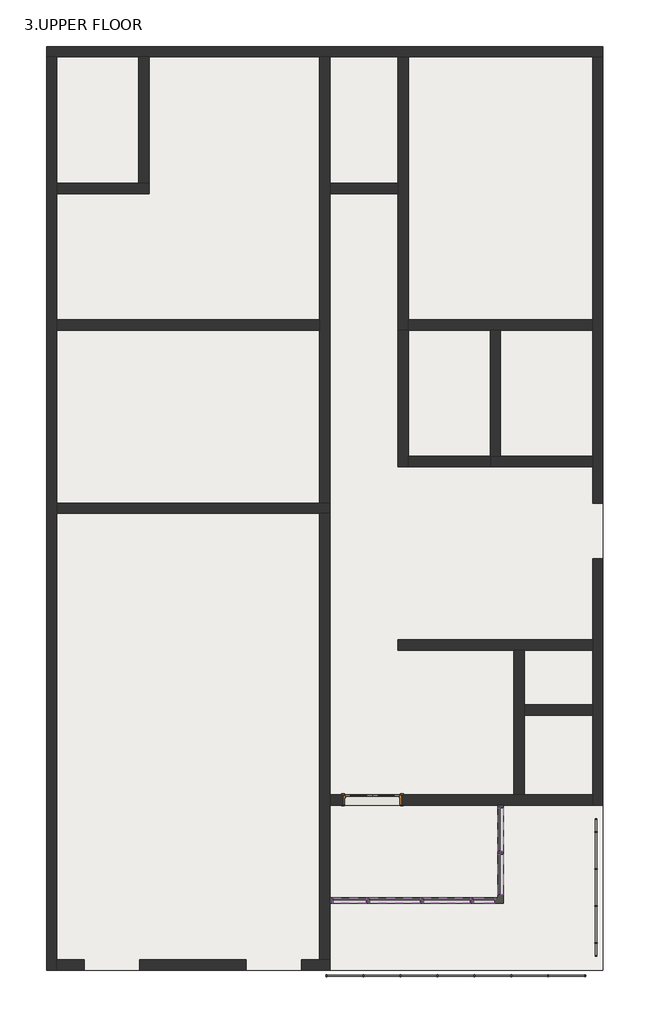
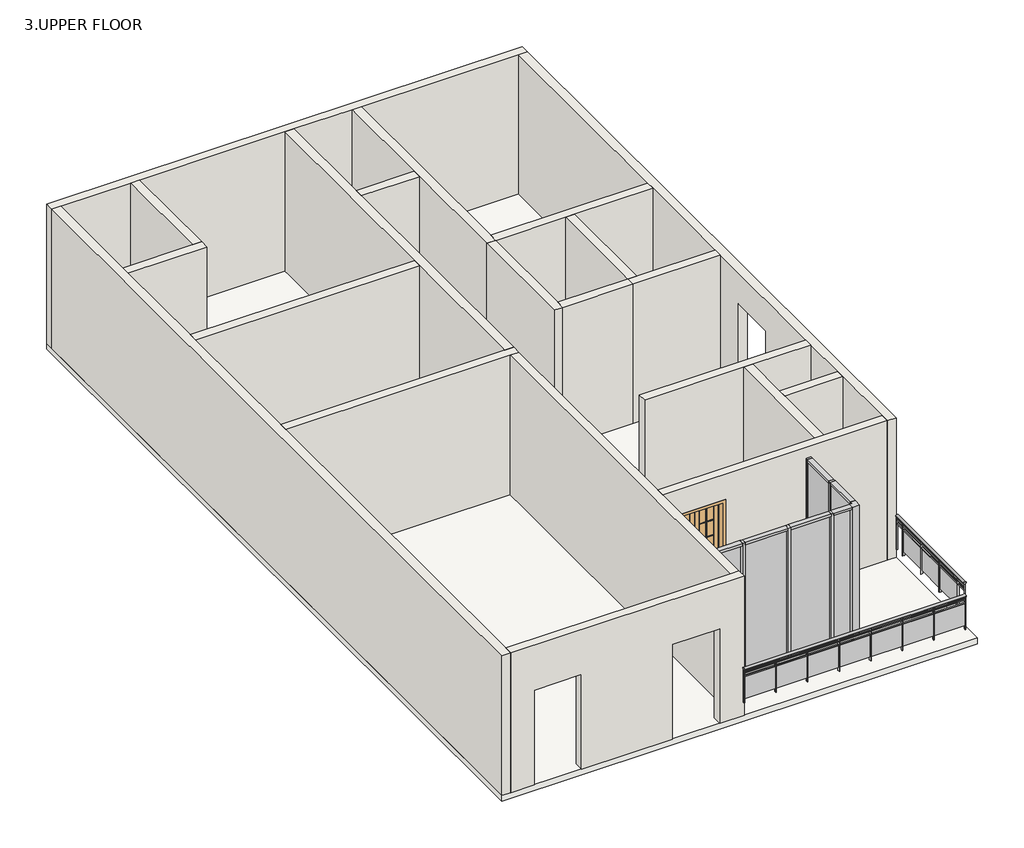
# One storey: 21 walls, 19 members, 6 plates, 2 railings, 1 door, 1 slab.
"""IFC4 building model written with IfcOpenShell, lengths in millimetres."""

from ifc_helpers import new_model, si_unit, point, frame, origin, place, context, project, spatial, polyline, ellipse_curve, trimmed, outline, extrude, faceted_brep, transform, mapped, element, save
from ifc_brep_helpers import plane_surface, extruded_surface, advanced_brep
from components import door_interior_double_full_glass_wood_4_x_8_0c92ad92, member_693e8272, member_0ce7375f, member_58dfa4c6, member_05798353, member_3e299884, member_a8ebf488, member_6e66df9c, member_e4ba5a11, member_9cf8e2d9, system_panel_glazed_02167798, system_panel_glazed_3d2c66d7, system_panel_glazed_0d5058d0, system_panel_glazed_5332cc33, system_panel_glazed_aeaff5c2, system_panel_glazed_b03b416e

model = new_model("IFC4")

# Units and contexts
model_context = context("Model", 3, world=origin())
ifc_project = project(units=[si_unit("LENGTHUNIT", "METRE", prefix="MILLI")], contexts=[model_context])

# Site, building, storey
site = spatial("IfcSite", under=ifc_project)
building = spatial("IfcBuilding", under=site)
storey = spatial("IfcBuildingStorey", under=building, Name="3.UPPER FLOOR", Elevation=3750.0)

# Door
placement = place(None, origin())
door_interior_double_full_glass_wood_4_x_8_shape = door_interior_double_full_glass_wood_4_x_8_0c92ad92(model_context)
element("IfcDoor", 1, ObjectType="Door-Interior-Double-Full Glass-Wood : 4' x 8'", at=placement, inside=storey, context=model_context, shape_type="MappedRepresentation", body=[
    mapped(door_interior_double_full_glass_wood_4_x_8_shape, transform((825.5463749, -5959.698087, 4359.6), x_axis=(1.0, 0.0, 0.0), y_axis=(0.0, 1.0, 0.0), z_axis=(0.0, 0.0, 1.0))),
])

# Members
member_shape = member_693e8272(model_context)
element("IfcMember", 2, ObjectType="L Corner Mullion : 5\" x 5\" Corner", at=placement, inside=storey, context=model_context, shape_type="MappedRepresentation", body=[
    mapped(member_shape, transform((3644.1463749, -8174.973087, 3750.0), x_axis=(1.0, 0.0, 0.0), y_axis=(0.0, -1.0, 0.0), z_axis=(0.0, 0.0, -1.0))),
])
member_2_shape = member_0ce7375f(model_context)
element("IfcMember", 3, ObjectType="Rectangular Mullion : 2.5\" x 5\" rectangular", at=placement, inside=storey, context=model_context, shape_type="MappedRepresentation", body=[
    mapped(member_2_shape, transform((-45.9536251, -8174.973087, 3750.0), x_axis=(0.0, 0.0, -1.0), y_axis=(0.0, -1.0, 0.0), z_axis=(-1.0, 0.0, 0.0))),
])
member_3_shape = member_58dfa4c6(model_context)
element("IfcMember", 4, ObjectType="Rectangular Mullion : 2.5\" x 5\" rectangular", at=placement, inside=storey, context=model_context, shape_type="MappedRepresentation", body=[
    mapped(member_3_shape, transform((730.5463749, -8174.973087, 3750.0), x_axis=(1.0, 0.0, 0.0), y_axis=(0.0, -1.0, 0.0), z_axis=(0.0, 0.0, -1.0))),
])
element("IfcMember", 5, ObjectType="Rectangular Mullion : 2.5\" x 5\" rectangular", at=placement, inside=storey, context=model_context, shape_type="MappedRepresentation", body=[
    mapped(member_3_shape, transform((1910.5463749, -8174.973087, 3750.0), x_axis=(1.0, 0.0, 0.0), y_axis=(0.0, -1.0, 0.0), z_axis=(0.0, 0.0, -1.0))),
])
element("IfcMember", 6, ObjectType="Rectangular Mullion : 2.5\" x 5\" rectangular", at=placement, inside=storey, context=model_context, shape_type="MappedRepresentation", body=[
    mapped(member_3_shape, transform((3012.9463749, -8174.973087, 3750.0), x_axis=(1.0, 0.0, 0.0), y_axis=(0.0, -1.0, 0.0), z_axis=(0.0, 0.0, -1.0))),
])
element("IfcMember", 7, ObjectType="Rectangular Mullion : 2.5\" x 5\" rectangular", at=placement, inside=storey, context=model_context, shape_type="MappedRepresentation", body=[
    mapped(member_3_shape, transform((3644.1463749, -7126.073087, 3750.0), x_axis=(0.0, 1.0, 0.0), y_axis=(1.0, 0.0, 0.0), z_axis=(0.0, 0.0, -1.0))),
])
member_4_shape = member_05798353(model_context)
element("IfcMember", 8, ObjectType="Rectangular Mullion : 2.5\" x 5\" rectangular", at=placement, inside=storey, context=model_context, shape_type="MappedRepresentation", body=[
    mapped(member_4_shape, transform((762.2963749, -8174.973087, 3750.0), x_axis=(0.0, 0.0, -1.0), y_axis=(0.0, -1.0, 0.0), z_axis=(-1.0, 0.0, 0.0))),
])
member_5_shape = member_3e299884(model_context)
element("IfcMember", 9, ObjectType="Rectangular Mullion : 2.5\" x 5\" rectangular", at=placement, inside=storey, context=model_context, shape_type="MappedRepresentation", body=[
    mapped(member_5_shape, transform((1942.2963749, -8174.973087, 3750.0), x_axis=(0.0, 0.0, -1.0), y_axis=(0.0, -1.0, 0.0), z_axis=(-1.0, 0.0, 0.0))),
])
element("IfcMember", 10, ObjectType="Rectangular Mullion : 2.5\" x 5\" rectangular", at=placement, inside=storey, context=model_context, shape_type="MappedRepresentation", body=[
    mapped(member_2_shape, transform((698.7963749, -8174.973087, 7256.9820397), x_axis=(0.0, 0.0, 1.0), y_axis=(0.0, -1.0, 0.0), z_axis=(1.0, 0.0, 0.0))),
])
element("IfcMember", 11, ObjectType="Rectangular Mullion : 2.5\" x 5\" rectangular", at=placement, inside=storey, context=model_context, shape_type="MappedRepresentation", body=[
    mapped(member_4_shape, transform((1878.7963749, -8174.973087, 7256.9820397), x_axis=(0.0, 0.0, 1.0), y_axis=(0.0, -1.0, 0.0), z_axis=(1.0, 0.0, 0.0))),
])
element("IfcMember", 12, ObjectType="Rectangular Mullion : 2.5\" x 5\" rectangular", at=placement, inside=storey, context=model_context, shape_type="MappedRepresentation", body=[
    mapped(member_5_shape, transform((2981.1963749, -8174.973087, 7256.9820397), x_axis=(0.0, 0.0, 1.0), y_axis=(0.0, -1.0, 0.0), z_axis=(1.0, 0.0, 0.0))),
])
member_6_shape = member_a8ebf488(model_context)
element("IfcMember", 13, ObjectType="Rectangular Mullion : 2.5\" x 5\" rectangular", at=placement, inside=storey, context=model_context, shape_type="MappedRepresentation", body=[
    mapped(member_6_shape, transform((-109.4536251, -8174.973087, 7256.9820397), x_axis=(-1.0, 0.0, 0.0), y_axis=(0.0, -1.0, 0.0), z_axis=(0.0, 0.0, 1.0))),
])
element("IfcMember", 14, ObjectType="Rectangular Mullion : 2.5\" x 5\" rectangular", at=placement, inside=storey, context=model_context, shape_type="MappedRepresentation", body=[
    mapped(member_6_shape, transform((3644.1463749, -6077.173087, 3750.0), x_axis=(0.0, 1.0, 0.0), y_axis=(1.0, 0.0, 0.0), z_axis=(0.0, 0.0, -1.0))),
])
member_7_shape = member_6e66df9c(model_context)
element("IfcMember", 15, ObjectType="Rectangular Mullion : 2.5\" x 5\" rectangular", at=placement, inside=storey, context=model_context, shape_type="MappedRepresentation", body=[
    mapped(member_7_shape, transform((3644.1463749, -6140.673087, 7256.9820397), x_axis=(0.0, 0.0, 1.0), y_axis=(1.0, 0.0, 0.0), z_axis=(0.0, 1.0, 0.0))),
])
element("IfcMember", 16, ObjectType="Rectangular Mullion : 2.5\" x 5\" rectangular", at=placement, inside=storey, context=model_context, shape_type="MappedRepresentation", body=[
    mapped(member_7_shape, transform((3644.1463749, -7094.323087, 3750.0), x_axis=(0.0, 0.0, -1.0), y_axis=(1.0, 0.0, 0.0), z_axis=(0.0, -1.0, 0.0))),
])
member_8_shape = member_e4ba5a11(model_context)
element("IfcMember", 17, ObjectType="Rectangular Mullion : 2.5\" x 5\" rectangular", at=placement, inside=storey, context=model_context, shape_type="MappedRepresentation", body=[
    mapped(member_8_shape, transform((3517.1463749, -8174.973087, 7256.9820397), x_axis=(0.0, 0.0, 1.0), y_axis=(0.0, -1.0, 0.0), z_axis=(1.0, 0.0, 0.0))),
])
element("IfcMember", 18, ObjectType="Rectangular Mullion : 2.5\" x 5\" rectangular", at=placement, inside=storey, context=model_context, shape_type="MappedRepresentation", body=[
    mapped(member_8_shape, transform((3044.6963749, -8174.973087, 3750.0), x_axis=(0.0, 0.0, -1.0), y_axis=(0.0, -1.0, 0.0), z_axis=(-1.0, 0.0, 0.0))),
])
member_9_shape = member_9cf8e2d9(model_context)
element("IfcMember", 19, ObjectType="Rectangular Mullion : 2.5\" x 5\" rectangular", at=placement, inside=storey, context=model_context, shape_type="MappedRepresentation", body=[
    mapped(member_9_shape, transform((3644.1463749, -8047.973087, 3750.0), x_axis=(0.0, 0.0, -1.0), y_axis=(1.0, 0.0, 0.0), z_axis=(0.0, -1.0, 0.0))),
])
element("IfcMember", 20, ObjectType="Rectangular Mullion : 2.5\" x 5\" rectangular", at=placement, inside=storey, context=model_context, shape_type="MappedRepresentation", body=[
    mapped(member_9_shape, transform((3644.1463749, -7157.823087, 7256.9820397), x_axis=(0.0, 0.0, 1.0), y_axis=(1.0, 0.0, 0.0), z_axis=(0.0, 1.0, 0.0))),
])

# Plates
system_panel_glazed_shape = system_panel_glazed_02167798(model_context)
element("IfcPlate", 21, ObjectType="System Panel : Glazed", at=placement, inside=storey, context=model_context, shape_type="MappedRepresentation", body=[
    mapped(system_panel_glazed_shape, transform((326.4213749, -8174.973087, 3813.5), x_axis=(1.0, 0.0, 0.0), y_axis=(0.0, 1.0, 0.0), z_axis=(0.0, 0.0, 1.0))),
])
system_panel_glazed_2_shape = system_panel_glazed_3d2c66d7(model_context)
element("IfcPlate", 22, ObjectType="System Panel : Glazed", at=placement, inside=storey, context=model_context, shape_type="MappedRepresentation", body=[
    mapped(system_panel_glazed_2_shape, transform((1320.5463749, -8174.973087, 3813.5), x_axis=(1.0, 0.0, 0.0), y_axis=(0.0, 1.0, 0.0), z_axis=(0.0, 0.0, 1.0))),
])
system_panel_glazed_3_shape = system_panel_glazed_0d5058d0(model_context)
element("IfcPlate", 23, ObjectType="System Panel : Glazed", at=placement, inside=storey, context=model_context, shape_type="MappedRepresentation", body=[
    mapped(system_panel_glazed_3_shape, transform((2461.7463749, -8174.973087, 3813.5), x_axis=(1.0, 0.0, 0.0), y_axis=(0.0, 1.0, 0.0), z_axis=(0.0, 0.0, 1.0))),
])
system_panel_glazed_4_shape = system_panel_glazed_5332cc33(model_context)
element("IfcPlate", 24, ObjectType="System Panel : Glazed", at=placement, inside=storey, context=model_context, shape_type="MappedRepresentation", body=[
    mapped(system_panel_glazed_4_shape, transform((3644.1463749, -6617.498087, 3813.5), x_axis=(0.0, 1.0, 0.0), y_axis=(-1.0, 0.0, 0.0), z_axis=(0.0, 0.0, 1.0))),
])
system_panel_glazed_5_shape = system_panel_glazed_aeaff5c2(model_context)
element("IfcPlate", 25, ObjectType="System Panel : Glazed", at=placement, inside=storey, context=model_context, shape_type="MappedRepresentation", body=[
    mapped(system_panel_glazed_5_shape, transform((3280.9213749, -8174.973087, 3813.5), x_axis=(1.0, 0.0, 0.0), y_axis=(0.0, 1.0, 0.0), z_axis=(0.0, 0.0, 1.0))),
])
system_panel_glazed_6_shape = system_panel_glazed_b03b416e(model_context)
element("IfcPlate", 26, ObjectType="System Panel : Glazed", at=placement, inside=storey, context=model_context, shape_type="MappedRepresentation", body=[
    mapped(system_panel_glazed_6_shape, transform((3644.1463749, -7602.898087, 3813.5), x_axis=(0.0, 1.0, 0.0), y_axis=(-1.0, 0.0, 0.0), z_axis=(0.0, 0.0, 1.0))),
])

# Railings
element("IfcRailing", 27, ObjectType="Glass Panel - Bottom Fill", at=placement, inside=storey, context=model_context, shape_type="SolidModel", body=[
    advanced_brep(
    [(5512.9463749, -9866.673087, 5121.6), (5512.9463749, -9790.473087, 5121.6), (-189.4536251, -9866.673087, 5121.6), (-189.4536251, -9790.473087, 5121.6)],
    [
        (0, 1, ellipse_curve(frame((5512.9463749, -9828.573087, 5121.6), z_axis=(1.0, 0.0, 0.0), x_axis=(0.0, 1.0, 0.0)), 38.1, 28.575)),
        (1, 0, ellipse_curve(frame((5512.9463749, -9828.573087, 5121.6), z_axis=(1.0, 0.0, 0.0), x_axis=(0.0, 1.0, 0.0)), 38.1, 28.575)),
        (2, 3, ellipse_curve(frame((-189.4536251, -9828.573087, 5121.6), z_axis=(-1.0, 0.0, 0.0), x_axis=(0.0, 1.0, 0.0)), 38.1, 28.575)),
        (3, 2, ellipse_curve(frame((-189.4536251, -9828.573087, 5121.6), z_axis=(-1.0, 0.0, 0.0), x_axis=(0.0, 1.0, 0.0)), 38.1, 28.575)),
        (0, 2),
        (3, 1),
    ],
    [
        plane_surface(frame((5512.9463749, -9828.573087, 5121.6), z_axis=(1.0, 0.0, 0.0), x_axis=(0.0, -1.0, 0.0))),
        plane_surface(frame((-189.4536251, -9828.573087, 5121.6), z_axis=(-1.0, 0.0, 0.0), x_axis=(0.0, -1.0, 0.0))),
        extruded_surface(trimmed(ellipse_curve(frame((-189.4536251, -9828.573087, 5121.6), z_axis=(1.0, 0.0, 0.0), x_axis=(0.0, 1.0, 0.0)), 38.1, 28.575), [point((-189.4536251, -9866.673087, 5121.6))], [point((-189.4536251, -9790.473087, 5121.6))], True, "CARTESIAN"), (5702.4, 0.0, 0.0), 5702.4),
        extruded_surface(trimmed(ellipse_curve(frame((-189.4536251, -9828.573087, 5121.6), z_axis=(1.0, 0.0, 0.0), x_axis=(0.0, 1.0, 0.0)), 38.1, 28.575), [point((-189.4536251, -9790.473087, 5121.6))], [point((-189.4536251, -9866.673087, 5121.6))], True, "CARTESIAN"), (5702.4, 0.0, 0.0), 5702.4),
    ],
    [
        (0, [[1, 2]]),
        (1, [[3, 4]]),
        (2, [[-1, 5, -4, 6]]),
        (3, [[-2, -6, -3, -5]]),
    ],
),
    extrude(outline(polyline([(5512.9463749, -9815.873087), (5512.9463749, -9841.273087), (-189.4536251, -9841.273087), (-189.4536251, -9815.873087), (5512.9463749, -9815.873087)])), frame((0.0, 0.0, 5007.3), z_axis=(0.0, 0.0, 1.0), x_axis=(1.0, 0.0, 0.0)), (0.0, 0.0, 1.0), 25.4),
    extrude(outline(polyline([(5512.9463749, -9815.873087), (5512.9463749, -9841.273087), (-189.4536251, -9841.273087), (-189.4536251, -9815.873087), (5512.9463749, -9815.873087)])), frame((0.0, 0.0, 4905.7), z_axis=(0.0, 0.0, 1.0), x_axis=(1.0, 0.0, 0.0)), (0.0, 0.0, 1.0), 25.4),
    extrude(outline(polyline([(-176.7036251, -9803.173087), (-176.7036251, -9853.973087), (-189.4036251, -9853.973087), (-189.4036251, -9803.173087), (-176.7036251, -9803.173087)])), frame((0.0, 0.0, 4207.2), z_axis=(0.0, 0.0, 1.0), x_axis=(1.0, 0.0, 0.0)), (0.0, 0.0, 1.0), 885.825),
    extrude(outline(polyline([(629.7463749, -9835.108244), (-183.0536251, -9835.108244), (-183.0536251, -9828.758244), (629.7463749, -9828.758244), (629.7463749, -9835.108244)])), frame((0.0, 0.0, 4308.8), z_axis=(0.0, 0.0, 1.0), x_axis=(1.0, 0.0, 0.0)), (0.0, 0.0, 1.0), 596.9),
    extrude(outline(polyline([(636.0963749, -9803.173087), (636.0963749, -9853.973087), (623.3963749, -9853.973087), (623.3963749, -9803.173087), (636.0963749, -9803.173087)])), frame((0.0, 0.0, 4207.2), z_axis=(0.0, 0.0, 1.0), x_axis=(1.0, 0.0, 0.0)), (0.0, 0.0, 1.0), 885.825),
    extrude(outline(polyline([(1442.5463749, -9835.108244), (629.7463749, -9835.108244), (629.7463749, -9828.758244), (1442.5463749, -9828.758244), (1442.5463749, -9835.108244)])), frame((0.0, 0.0, 4308.8), z_axis=(0.0, 0.0, 1.0), x_axis=(1.0, 0.0, 0.0)), (0.0, 0.0, 1.0), 596.9),
    extrude(outline(polyline([(1448.8963749, -9803.173087), (1448.8963749, -9853.973087), (1436.1963749, -9853.973087), (1436.1963749, -9803.173087), (1448.8963749, -9803.173087)])), frame((0.0, 0.0, 4207.2), z_axis=(0.0, 0.0, 1.0), x_axis=(1.0, 0.0, 0.0)), (0.0, 0.0, 1.0), 885.825),
    extrude(outline(polyline([(2255.3463749, -9835.108244), (1442.5463749, -9835.108244), (1442.5463749, -9828.758244), (2255.3463749, -9828.758244), (2255.3463749, -9835.108244)])), frame((0.0, 0.0, 4308.8), z_axis=(0.0, 0.0, 1.0), x_axis=(1.0, 0.0, 0.0)), (0.0, 0.0, 1.0), 596.9),
    extrude(outline(polyline([(2261.6963749, -9803.173087), (2261.6963749, -9853.973087), (2248.9963749, -9853.973087), (2248.9963749, -9803.173087), (2261.6963749, -9803.173087)])), frame((0.0, 0.0, 4207.2), z_axis=(0.0, 0.0, 1.0), x_axis=(1.0, 0.0, 0.0)), (0.0, 0.0, 1.0), 885.825),
    extrude(outline(polyline([(3068.1463749, -9835.108244), (2255.3463749, -9835.108244), (2255.3463749, -9828.758244), (3068.1463749, -9828.758244), (3068.1463749, -9835.108244)])), frame((0.0, 0.0, 4308.8), z_axis=(0.0, 0.0, 1.0), x_axis=(1.0, 0.0, 0.0)), (0.0, 0.0, 1.0), 596.9),
    extrude(outline(polyline([(3074.4963749, -9803.173087), (3074.4963749, -9853.973087), (3061.7963749, -9853.973087), (3061.7963749, -9803.173087), (3074.4963749, -9803.173087)])), frame((0.0, 0.0, 4207.2), z_axis=(0.0, 0.0, 1.0), x_axis=(1.0, 0.0, 0.0)), (0.0, 0.0, 1.0), 885.825),
    extrude(outline(polyline([(3880.9463749, -9835.108244), (3068.1463749, -9835.108244), (3068.1463749, -9828.758244), (3880.9463749, -9828.758244), (3880.9463749, -9835.108244)])), frame((0.0, 0.0, 4308.8), z_axis=(0.0, 0.0, 1.0), x_axis=(1.0, 0.0, 0.0)), (0.0, 0.0, 1.0), 596.9),
    extrude(outline(polyline([(3887.2963749, -9803.173087), (3887.2963749, -9853.973087), (3874.5963749, -9853.973087), (3874.5963749, -9803.173087), (3887.2963749, -9803.173087)])), frame((0.0, 0.0, 4207.2), z_axis=(0.0, 0.0, 1.0), x_axis=(1.0, 0.0, 0.0)), (0.0, 0.0, 1.0), 885.825),
    extrude(outline(polyline([(4693.7463749, -9835.108244), (3880.9463749, -9835.108244), (3880.9463749, -9828.758244), (4693.7463749, -9828.758244), (4693.7463749, -9835.108244)])), frame((0.0, 0.0, 4308.8), z_axis=(0.0, 0.0, 1.0), x_axis=(1.0, 0.0, 0.0)), (0.0, 0.0, 1.0), 596.9),
    extrude(outline(polyline([(4700.0963749, -9803.173087), (4700.0963749, -9853.973087), (4687.3963749, -9853.973087), (4687.3963749, -9803.173087), (4700.0963749, -9803.173087)])), frame((0.0, 0.0, 4207.2), z_axis=(0.0, 0.0, 1.0), x_axis=(1.0, 0.0, 0.0)), (0.0, 0.0, 1.0), 885.825),
    extrude(outline(polyline([(5506.5463749, -9835.108244), (4693.7463749, -9835.108244), (4693.7463749, -9828.758244), (5506.5463749, -9828.758244), (5506.5463749, -9835.108244)])), frame((0.0, 0.0, 4308.8), z_axis=(0.0, 0.0, 1.0), x_axis=(1.0, 0.0, 0.0)), (0.0, 0.0, 1.0), 596.9),
    extrude(outline(polyline([(5512.8963749, -9803.173087), (5512.8963749, -9853.973087), (5500.1963749, -9853.973087), (5500.1963749, -9803.173087), (5512.8963749, -9803.173087)])), frame((0.0, 0.0, 4207.2), z_axis=(0.0, 0.0, 1.0), x_axis=(1.0, 0.0, 0.0)), (0.0, 0.0, 1.0), 885.825),
    extrude(outline(polyline([(-176.7536251, -9819.048087), (-176.7536251, -9838.098087), (-195.8036251, -9838.098087), (-195.8036251, -9819.048087), (-176.7536251, -9819.048087)])), frame((0.0, 0.0, 4207.2), z_axis=(0.0, 0.0, 1.0), x_axis=(1.0, 0.0, 0.0)), (0.0, 0.0, 1.0), 885.825),
    extrude(outline(polyline([(5519.2963749, -9819.048087), (5519.2963749, -9838.098087), (5500.2463749, -9838.098087), (5500.2463749, -9819.048087), (5519.2963749, -9819.048087)])), frame((0.0, 0.0, 4207.2), z_axis=(0.0, 0.0, 1.0), x_axis=(1.0, 0.0, 0.0)), (0.0, 0.0, 1.0), 885.825),
])
element("IfcRailing", 28, ObjectType="Glass Panel - Bottom Fill", at=placement, inside=storey, context=model_context, shape_type="SolidModel", body=[
    advanced_brep(
    [(5783.4463749, -6381.973087, 5121.6), (5707.2463749, -6381.973087, 5121.6), (5783.4463749, -9398.773087, 5121.6), (5707.2463749, -9398.773087, 5121.6)],
    [
        (0, 1, ellipse_curve(frame((5745.3463749, -6381.973087, 5121.6), z_axis=(0.0, 1.0, 0.0), x_axis=(-1.0, 0.0, 0.0)), 38.1, 28.575)),
        (1, 0, ellipse_curve(frame((5745.3463749, -6381.973087, 5121.6), z_axis=(0.0, 1.0, 0.0), x_axis=(-1.0, 0.0, 0.0)), 38.1, 28.575)),
        (2, 3, ellipse_curve(frame((5745.3463749, -9398.773087, 5121.6), z_axis=(0.0, -1.0, 0.0), x_axis=(-1.0, 0.0, 0.0)), 38.1, 28.575)),
        (3, 2, ellipse_curve(frame((5745.3463749, -9398.773087, 5121.6), z_axis=(0.0, -1.0, 0.0), x_axis=(-1.0, 0.0, 0.0)), 38.1, 28.575)),
        (0, 2),
        (3, 1),
    ],
    [
        plane_surface(frame((5745.3463749, -6381.973087, 5121.6), z_axis=(0.0, 1.0, 0.0), x_axis=(0.0, 0.0, -1.0))),
        plane_surface(frame((5745.3463749, -9398.773087, 5121.6), z_axis=(0.0, -1.0, 0.0), x_axis=(0.0, 0.0, -1.0))),
        extruded_surface(trimmed(ellipse_curve(frame((5745.3463749, -9398.773087, 5121.6), z_axis=(0.0, 1.0, 0.0), x_axis=(-1.0, 0.0, 0.0)), 38.1, 28.575), [point((5783.4463749, -9398.773087, 5121.6))], [point((5707.2463749, -9398.773087, 5121.6))], True, "CARTESIAN"), (0.0, 3016.7999999999993, 0.0), 3016.7999999999993),
        extruded_surface(trimmed(ellipse_curve(frame((5745.3463749, -9398.773087, 5121.6), z_axis=(0.0, 1.0, 0.0), x_axis=(-1.0, 0.0, 0.0)), 38.1, 28.575), [point((5707.2463749, -9398.773087, 5121.6))], [point((5783.4463749, -9398.773087, 5121.6))], True, "CARTESIAN"), (0.0, 3016.7999999999993, 0.0), 3016.7999999999993),
    ],
    [
        (0, [[1, 2]]),
        (1, [[3, 4]]),
        (2, [[-1, 5, -4, 6]]),
        (3, [[-2, -6, -3, -5]]),
    ],
),
    extrude(outline(polyline([(5732.6463749, -6381.973087), (5758.0463749, -6381.973087), (5758.0463749, -9398.773087), (5732.6463749, -9398.773087), (5732.6463749, -6381.973087)])), frame((0.0, 0.0, 5007.3), z_axis=(0.0, 0.0, 1.0), x_axis=(1.0, 0.0, 0.0)), (0.0, 0.0, 1.0), 25.4),
    extrude(outline(polyline([(5732.6463749, -6381.973087), (5758.0463749, -6381.973087), (5758.0463749, -9398.773087), (5732.6463749, -9398.773087), (5732.6463749, -6381.973087)])), frame((0.0, 0.0, 4905.7), z_axis=(0.0, 0.0, 1.0), x_axis=(1.0, 0.0, 0.0)), (0.0, 0.0, 1.0), 25.4),
    extrude(outline(polyline([(5719.9463749, -9103.223087), (5770.7463749, -9103.223087), (5770.7463749, -9115.923087), (5719.9463749, -9115.923087), (5719.9463749, -9103.223087)])), frame((0.0, 0.0, 4207.2), z_axis=(0.0, 0.0, 1.0), x_axis=(1.0, 0.0, 0.0)), (0.0, 0.0, 1.0), 885.825),
    extrude(outline(polyline([(5751.8815319, -8296.773087), (5751.8815319, -9109.573087), (5745.5315319, -9109.573087), (5745.5315319, -8296.773087), (5751.8815319, -8296.773087)])), frame((0.0, 0.0, 4308.8), z_axis=(0.0, 0.0, 1.0), x_axis=(1.0, 0.0, 0.0)), (0.0, 0.0, 1.0), 596.9),
    extrude(outline(polyline([(5719.9463749, -8290.423087), (5770.7463749, -8290.423087), (5770.7463749, -8303.123087), (5719.9463749, -8303.123087), (5719.9463749, -8290.423087)])), frame((0.0, 0.0, 4207.2), z_axis=(0.0, 0.0, 1.0), x_axis=(1.0, 0.0, 0.0)), (0.0, 0.0, 1.0), 885.825),
    extrude(outline(polyline([(5751.8815319, -7483.973087), (5751.8815319, -8296.773087), (5745.5315319, -8296.773087), (5745.5315319, -7483.973087), (5751.8815319, -7483.973087)])), frame((0.0, 0.0, 4308.8), z_axis=(0.0, 0.0, 1.0), x_axis=(1.0, 0.0, 0.0)), (0.0, 0.0, 1.0), 596.9),
    extrude(outline(polyline([(5719.9463749, -7477.623087), (5770.7463749, -7477.623087), (5770.7463749, -7490.323087), (5719.9463749, -7490.323087), (5719.9463749, -7477.623087)])), frame((0.0, 0.0, 4207.2), z_axis=(0.0, 0.0, 1.0), x_axis=(1.0, 0.0, 0.0)), (0.0, 0.0, 1.0), 885.825),
    extrude(outline(polyline([(5751.8815319, -6671.173087), (5751.8815319, -7483.973087), (5745.5315319, -7483.973087), (5745.5315319, -6671.173087), (5751.8815319, -6671.173087)])), frame((0.0, 0.0, 4308.8), z_axis=(0.0, 0.0, 1.0), x_axis=(1.0, 0.0, 0.0)), (0.0, 0.0, 1.0), 596.9),
    extrude(outline(polyline([(5719.9463749, -6664.823087), (5770.7463749, -6664.823087), (5770.7463749, -6677.523087), (5719.9463749, -6677.523087), (5719.9463749, -6664.823087)])), frame((0.0, 0.0, 4207.2), z_axis=(0.0, 0.0, 1.0), x_axis=(1.0, 0.0, 0.0)), (0.0, 0.0, 1.0), 885.825),
    extrude(outline(polyline([(5735.8213749, -9386.073087), (5754.8713749, -9386.073087), (5754.8713749, -9405.123087), (5735.8213749, -9405.123087), (5735.8213749, -9386.073087)])), frame((0.0, 0.0, 4207.2), z_axis=(0.0, 0.0, 1.0), x_axis=(1.0, 0.0, 0.0)), (0.0, 0.0, 1.0), 885.825),
    extrude(outline(polyline([(5735.8213749, -6375.623087), (5754.8713749, -6375.623087), (5754.8713749, -6394.673087), (5735.8213749, -6394.673087), (5735.8213749, -6375.623087)])), frame((0.0, 0.0, 4207.2), z_axis=(0.0, 0.0, 1.0), x_axis=(1.0, 0.0, 0.0)), (0.0, 0.0, 1.0), 885.825),
])

# Slab
element("IfcSlab", 29, ObjectType="6\" floor", at=placement, inside=storey, context=model_context, shape_type="SweptSolid", body=[
    extrude(outline(polyline([(-6341.6536251, 10590.826913), (5897.7463749, 10590.826913), (5897.7463749, -9703.573087), (-6341.6536251, -9703.573087), (-6341.6536251, 10590.826913)])), frame((0.0, 0.0, 3597.6), z_axis=(0.0, 0.0, 1.0), x_axis=(1.0, 0.0, 0.0)), (0.0, 0.0, 1.0), 152.4),
])

# Walls
element("IfcWall", 30, ObjectType="9\" wall", at=placement, inside=storey, context=model_context, shape_type="Brep", body=[
    faceted_brep([(-6341.6536251, 10362.226913, 3750.0), (-6113.0536251, 10362.226913, 3750.0), (-4313.0536251, 10362.226913, 3750.0), (-4084.4536251, 10362.226913, 3750.0), (-338.0536251, 10362.226913, 3750.0), (-109.4536251, 10362.226913, 3750.0), (1390.5463749, 10362.226913, 3750.0), (1619.1463749, 10362.226913, 3750.0), (5669.1463749, 10362.226913, 3750.0), (5897.7463749, 10362.226913, 3750.0), (5897.7463749, 10362.226913, 7547.6), (5669.1463749, 10362.226913, 7547.6), (1619.1463749, 10362.226913, 7547.6), (1390.5463749, 10362.226913, 7547.6), (-109.4536251, 10362.226913, 7547.6), (-338.0536251, 10362.226913, 7547.6), (-4084.4536251, 10362.226913, 7547.6), (-4313.0536251, 10362.226913, 7547.6), (-6113.0536251, 10362.226913, 7547.6), (-6341.6536251, 10362.226913, 7547.6), (-6341.6536251, 10590.826913, 3750.0), (-6341.6536251, 10590.826913, 7547.6), (5897.7463749, 10590.826913, 7547.6), (5897.7463749, 10590.826913, 3750.0)], [[[0, 1, 2, 3, 4, 5, 6, 7, 8, 9, 10, 11, 12, 13, 14, 15, 16, 17, 18, 19]], [[20, 21, 22, 23]], [[9, 8, 7, 6, 5, 4, 3, 2, 1, 0, 20, 23]], [[0, 19, 21, 20]], [[10, 9, 23, 22]], [[19, 18, 17, 16, 15, 14, 13, 12, 11, 10, 22, 21]]]),
])
element("IfcWall", 31, ObjectType="9\" wall", at=placement, inside=storey, context=model_context, shape_type="Brep", body=[
    faceted_brep([(-6113.0536251, -9703.573087, 3750.0), (-6113.0536251, -9474.973087, 3750.0), (-6113.0536251, 330.026913, 3750.0), (-6113.0536251, 558.626913, 3750.0), (-6113.0536251, 4358.626913, 3750.0), (-6113.0536251, 4587.226913, 3750.0), (-6113.0536251, 7358.626913, 3750.0), (-6113.0536251, 7587.226913, 3750.0), (-6113.0536251, 10362.226913, 3750.0), (-6113.0536251, 10362.226913, 7547.6), (-6113.0536251, 7587.226913, 7547.6), (-6113.0536251, 7358.626913, 7547.6), (-6113.0536251, 4587.226913, 7547.6), (-6113.0536251, 4358.626913, 7547.6), (-6113.0536251, 558.626913, 7547.6), (-6113.0536251, 330.026913, 7547.6), (-6113.0536251, -9474.973087, 7547.6), (-6113.0536251, -9703.573087, 7547.6), (-6341.6536251, -9703.573087, 3750.0), (-6341.6536251, -9703.573087, 7547.6), (-6341.6536251, -6077.173087, 7547.6), (-6341.6536251, 10362.226913, 7547.6), (-6341.6536251, 10362.226913, 3750.0)], [[[0, 1, 2, 3, 4, 5, 6, 7, 8, 9, 10, 11, 12, 13, 14, 15, 16, 17]], [[18, 19, 20, 21, 22]], [[8, 7, 6, 5, 4, 3, 2, 1, 0, 18, 22]], [[9, 8, 22, 21]], [[0, 17, 19, 18]], [[17, 16, 15, 14, 13, 12, 11, 10, 9, 21, 20, 19]]]),
])
element("IfcWall", 32, ObjectType="9\" wall", at=placement, inside=storey, context=model_context, shape_type="Brep", body=[
    faceted_brep([(-6113.0536251, 7358.626913, 3750.0), (-4084.4536251, 7358.626913, 3750.0), (-4084.4536251, 7358.626913, 7547.6), (-6113.0536251, 7358.626913, 7547.6), (-6113.0536251, 7587.226913, 3750.0), (-6113.0536251, 7587.226913, 7547.6), (-4313.0536251, 7587.226913, 7547.6), (-4084.4536251, 7587.226913, 7547.6), (-4084.4536251, 7587.226913, 3750.0), (-4313.0536251, 7587.226913, 3750.0)], [[[0, 1, 2, 3]], [[4, 5, 6, 7, 8, 9]], [[1, 0, 4, 9, 8]], [[0, 3, 5, 4]], [[2, 1, 8, 7]], [[3, 2, 7, 6, 5]]]),
])
element("IfcWall", 33, ObjectType="9\" wall", at=placement, inside=storey, context=model_context, shape_type="SweptSolid", body=[
    extrude(outline(polyline([(-4084.4536251, 10362.226913), (-4084.4536251, 7587.226913), (-4313.0536251, 7587.226913), (-4313.0536251, 10362.226913), (-4084.4536251, 10362.226913)])), frame((0.0, 0.0, 3750.0), z_axis=(0.0, 0.0, 1.0), x_axis=(1.0, 0.0, 0.0)), (0.0, 0.0, 1.0), 3797.6),
])
element("IfcWall", 34, ObjectType="9\" wall", at=placement, inside=storey, context=model_context, shape_type="SweptSolid", body=[
    extrude(outline(polyline([(-338.0536251, 4358.626913), (-6113.0536251, 4358.626913), (-6113.0536251, 4587.226913), (-338.0536251, 4587.226913), (-338.0536251, 4358.626913)])), frame((0.0, 0.0, 3750.0), z_axis=(0.0, 0.0, 1.0), x_axis=(1.0, 0.0, 0.0)), (0.0, 0.0, 1.0), 3797.6),
])
element("IfcWall", 35, ObjectType="9\" wall", at=placement, inside=storey, context=model_context, shape_type="Brep", body=[
    faceted_brep([(-109.4536251, 558.626913, 3750.0), (-109.4536251, 7358.626913, 3750.0), (-109.4536251, 7587.226913, 3750.0), (-109.4536251, 10362.226913, 3750.0), (-109.4536251, 10362.226913, 7547.6), (-109.4536251, 7587.226913, 7547.6), (-109.4536251, 7358.626913, 7547.6), (-109.4536251, 558.626913, 7547.6), (-338.0536251, 558.626913, 3750.0), (-338.0536251, 558.626913, 7547.6), (-338.0536251, 4358.626913, 7547.6), (-338.0536251, 4587.226913, 7547.6), (-338.0536251, 10362.226913, 7547.6), (-338.0536251, 10362.226913, 3750.0), (-338.0536251, 4587.226913, 3750.0), (-338.0536251, 4358.626913, 3750.0)], [[[0, 1, 2, 3, 4, 5, 6, 7]], [[8, 9, 10, 11, 12, 13, 14, 15]], [[3, 2, 1, 0, 8, 15, 14, 13]], [[4, 3, 13, 12]], [[0, 7, 9, 8]], [[7, 6, 5, 4, 12, 11, 10, 9]]]),
])
element("IfcWall", 36, ObjectType="9\" wall", at=placement, inside=storey, context=model_context, shape_type="Brep", body=[
    faceted_brep([(-6113.0536251, 330.026913, 3750.0), (-338.0536251, 330.026913, 3750.0), (-109.4536251, 330.026913, 3750.0), (-109.4536251, 330.026913, 7547.6), (-338.0536251, 330.026913, 7547.6), (-6113.0536251, 330.026913, 7547.6), (-6113.0536251, 558.626913, 3750.0), (-6113.0536251, 558.626913, 7547.6), (-338.0536251, 558.626913, 7547.6), (-109.4536251, 558.626913, 7547.6), (-109.4536251, 558.626913, 3750.0), (-338.0536251, 558.626913, 3750.0)], [[[0, 1, 2, 3, 4, 5]], [[6, 7, 8, 9, 10, 11]], [[2, 1, 0, 6, 11, 10]], [[0, 5, 7, 6]], [[3, 2, 10, 9]], [[5, 4, 3, 9, 8, 7]]]),
])
element("IfcWall", 37, ObjectType="9\" wall", at=placement, inside=storey, context=model_context, shape_type="Brep", body=[
    faceted_brep([(-109.4536251, -9703.573087, 3750.0), (-109.4536251, -9703.573087, 7547.6), (-6113.0536251, -9703.573087, 7547.6), (-6113.0536251, -9703.573087, 3750.0), (-5513.0536251, -9703.573087, 3750.0), (-5513.0536251, -9703.573087, 6324.1896655), (-4293.8536251, -9703.573087, 6324.1896655), (-4293.8536251, -9703.573087, 3750.0), (-1957.2536251, -9703.573087, 3750.0), (-1957.2536251, -9703.573087, 6324.1896655), (-738.0536251, -9703.573087, 6324.1896655), (-738.0536251, -9703.573087, 3750.0), (-109.4536251, -9474.973087, 7547.6), (-109.4536251, -9474.973087, 3750.0), (-338.0536251, -9474.973087, 3750.0), (-738.0536251, -9474.973087, 3750.0), (-738.0536251, -9474.973087, 6324.1896655), (-1957.2536251, -9474.973087, 6324.1896655), (-1957.2536251, -9474.973087, 3750.0), (-4293.8536251, -9474.973087, 3750.0), (-4293.8536251, -9474.973087, 6324.1896655), (-5513.0536251, -9474.973087, 6324.1896655), (-5513.0536251, -9474.973087, 3750.0), (-6113.0536251, -9474.973087, 3750.0), (-6113.0536251, -9474.973087, 7547.6), (-338.0536251, -9474.973087, 7547.6)], [[[0, 1, 2, 3, 4, 5, 6, 7, 8, 9, 10, 11]], [[12, 13, 14, 15, 16, 17, 18, 19, 20, 21, 22, 23, 24, 25]], [[13, 0, 11, 15, 14]], [[3, 23, 22, 4]], [[7, 19, 18, 8]], [[1, 0, 13, 12]], [[3, 2, 24, 23]], [[21, 5, 4, 22]], [[5, 21, 20, 6]], [[6, 20, 19, 7]], [[10, 16, 15, 11]], [[16, 10, 9, 17]], [[17, 9, 8, 18]], [[2, 1, 12, 25, 24]]]),
])
element("IfcWall", 38, ObjectType="9\" wall", at=placement, inside=storey, context=model_context, shape_type="Brep", body=[
    faceted_brep([(-109.4536251, -9474.973087, 3750.0), (-109.4536251, -6077.173087, 3750.0), (-109.4536251, -5848.573087, 3750.0), (-109.4536251, 330.026913, 3750.0), (-109.4536251, 330.026913, 7547.6), (-109.4536251, -5848.573087, 7547.6), (-109.4536251, -6077.173087, 7547.6), (-109.4536251, -9474.973087, 7547.6), (-338.0536251, -9474.973087, 3750.0), (-338.0536251, -9474.973087, 7547.6), (-338.0536251, 330.026913, 7547.6), (-338.0536251, 330.026913, 3750.0)], [[[0, 1, 2, 3, 4, 5, 6, 7]], [[8, 9, 10, 11]], [[3, 2, 1, 0, 8, 11]], [[0, 7, 9, 8]], [[4, 3, 11, 10]], [[7, 6, 5, 4, 10, 9]]]),
])
element("IfcWall", 39, ObjectType="9\" wall", at=placement, inside=storey, context=model_context, shape_type="Brep", body=[
    faceted_brep([(1390.5463749, 10362.226913, 3750.0), (1390.5463749, 7587.226913, 3750.0), (1390.5463749, 7358.626913, 3750.0), (1390.5463749, 4358.626913, 3750.0), (1390.5463749, 4358.626913, 7547.6), (1390.5463749, 7358.626913, 7547.6), (1390.5463749, 7587.226913, 7547.6), (1390.5463749, 10362.226913, 7547.6), (1619.1463749, 10362.226913, 3750.0), (1619.1463749, 10362.226913, 7547.6), (1619.1463749, 4587.226913, 7547.6), (1619.1463749, 4358.626913, 7547.6), (1619.1463749, 4358.626913, 3750.0), (1619.1463749, 4587.226913, 3750.0), (1615.5463749, 4358.626913, 3750.0), (1615.5463749, 4358.626913, 7547.6)], [[[0, 1, 2, 3, 4, 5, 6, 7]], [[8, 9, 10, 11, 12, 13]], [[3, 2, 1, 0, 8, 13, 12, 14]], [[0, 7, 9, 8]], [[4, 3, 14, 12, 11, 15]], [[7, 6, 5, 4, 15, 11, 10, 9]]]),
])
element("IfcWall", 40, ObjectType="9\" wall", at=placement, inside=storey, context=model_context, shape_type="SweptSolid", body=[
    extrude(outline(polyline([(-109.4536251, 7587.226913), (1390.5463749, 7587.226913), (1390.5463749, 7358.626913), (-109.4536251, 7358.626913), (-109.4536251, 7587.226913)])), frame((0.0, 0.0, 3750.0), z_axis=(0.0, 0.0, 1.0), x_axis=(1.0, 0.0, 0.0)), (0.0, 0.0, 1.0), 3797.6),
])
element("IfcWall", 41, ObjectType="9\" wall", at=placement, inside=storey, context=model_context, shape_type="Brep", body=[
    faceted_brep([(5669.1463749, 10362.226913, 7547.6), (5669.1463749, 10362.226913, 3750.0), (5669.1463749, 4587.226913, 3750.0), (5669.1463749, 4358.626913, 3750.0), (5669.1463749, 1583.626913, 3750.0), (5669.1463749, 1355.026913, 3750.0), (5669.1463749, 558.626913, 3750.0), (5669.1463749, 558.626913, 6707.7288504), (5669.1463749, -660.573087, 6707.7288504), (5669.1463749, -660.573087, 3750.0), (5669.1463749, -2444.973087, 3750.0), (5669.1463749, -2673.573087, 3750.0), (5669.1463749, -3873.573087, 3750.0), (5669.1463749, -4102.173087, 3750.0), (5669.1463749, -5848.573087, 3750.0), (5669.1463749, -6077.173087, 3750.0), (5669.1463749, -6077.173087, 7547.6), (5669.1463749, -5848.573087, 7547.6), (5669.1463749, -4102.173087, 7547.6), (5669.1463749, -3873.573087, 7547.6), (5669.1463749, -2673.573087, 7547.6), (5669.1463749, -2444.973087, 7547.6), (5669.1463749, 1355.026913, 7547.6), (5669.1463749, 1583.626913, 7547.6), (5669.1463749, 4358.626913, 7547.6), (5669.1463749, 4587.226913, 7547.6), (5897.7463749, 10362.226913, 3750.0), (5897.7463749, 10362.226913, 7547.6), (5897.7463749, -6077.173087, 7547.6), (5897.7463749, -6077.173087, 3750.0), (5897.7463749, -660.573087, 3750.0), (5897.7463749, -660.573087, 6707.7288504), (5897.7463749, 558.626913, 6707.7288504), (5897.7463749, 558.626913, 3750.0)], [[[0, 1, 2, 3, 4, 5, 6, 7, 8, 9, 10, 11, 12, 13, 14, 15, 16, 17, 18, 19, 20, 21, 22, 23, 24, 25]], [[26, 27, 28, 29, 30, 31, 32, 33]], [[1, 26, 33, 6, 5, 4, 3, 2]], [[29, 15, 14, 13, 12, 11, 10, 9, 30]], [[1, 0, 27, 26]], [[16, 15, 29, 28]], [[0, 25, 24, 23, 22, 21, 20, 19, 18, 17, 16, 28, 27]], [[32, 7, 6, 33]], [[7, 32, 31, 8]], [[8, 31, 30, 9]]]),
])
element("IfcWall", 42, ObjectType="9\" wall", at=placement, inside=storey, context=model_context, shape_type="Brep", body=[
    faceted_brep([(5669.1463749, 4587.226913, 3750.0), (1619.1463749, 4587.226913, 3750.0), (1619.1463749, 4587.226913, 7547.6), (5669.1463749, 4587.226913, 7547.6), (5669.1463749, 4358.626913, 3750.0), (5669.1463749, 4358.626913, 7547.6), (3644.1463749, 4358.626913, 7547.6), (3415.5463749, 4358.626913, 7547.6), (1619.1463749, 4358.626913, 7547.6), (1619.1463749, 4358.626913, 3750.0), (3415.5463749, 4358.626913, 3750.0), (3644.1463749, 4358.626913, 3750.0)], [[[0, 1, 2, 3]], [[4, 5, 6, 7, 8, 9, 10, 11]], [[1, 0, 4, 11, 10, 9]], [[2, 1, 9, 8]], [[0, 3, 5, 4]], [[3, 2, 8, 7, 6, 5]]]),
])
element("IfcWall", 43, ObjectType="9\" wall", at=placement, inside=storey, context=model_context, shape_type="Brep", body=[
    faceted_brep([(5669.1463749, 1583.626913, 3750.0), (3644.1463749, 1583.626913, 3750.0), (3415.5463749, 1583.626913, 3750.0), (3415.5463749, 1583.626913, 7547.6), (3644.1463749, 1583.626913, 7547.6), (5669.1463749, 1583.626913, 7547.6), (5669.1463749, 1355.026913, 3750.0), (5669.1463749, 1355.026913, 7547.6), (3415.5463749, 1355.026913, 7547.6), (3415.5463749, 1355.026913, 3750.0)], [[[0, 1, 2, 3, 4, 5]], [[6, 7, 8, 9]], [[2, 1, 0, 6, 9]], [[0, 5, 7, 6]], [[3, 2, 9, 8]], [[5, 4, 3, 8, 7]]]),
])
element("IfcWall", 44, ObjectType="9\" wall", at=placement, inside=storey, context=model_context, shape_type="SweptSolid", body=[
    extrude(outline(polyline([(3644.1463749, 4358.626913), (3644.1463749, 1583.626913), (3415.5463749, 1583.626913), (3415.5463749, 4358.626913), (3644.1463749, 4358.626913)])), frame((0.0, 0.0, 3750.0), z_axis=(0.0, 0.0, 1.0), x_axis=(1.0, 0.0, 0.0)), (0.0, 0.0, 1.0), 3797.6),
])
element("IfcWall", 45, ObjectType="9\" wall", at=placement, inside=storey, context=model_context, shape_type="Brep", body=[
    faceted_brep([(1386.9463749, 4358.626913, 3750.0), (1386.9463749, 1355.026913, 3750.0), (1386.9463749, 1355.026913, 7547.6), (1386.9463749, 4358.626913, 7547.6), (1615.5463749, 4358.626913, 3750.0), (1615.5463749, 4358.626913, 7547.6), (1615.5463749, 1583.626913, 7547.6), (1615.5463749, 1355.026913, 7547.6), (1615.5463749, 1355.026913, 3750.0), (1615.5463749, 1583.626913, 3750.0), (1390.5463749, 4358.626913, 3750.0), (1390.5463749, 4358.626913, 7547.6)], [[[0, 1, 2, 3]], [[4, 5, 6, 7, 8, 9]], [[1, 0, 10, 4, 9, 8]], [[0, 3, 11, 5, 4, 10]], [[2, 1, 8, 7]], [[3, 2, 7, 6, 5, 11]]]),
])
element("IfcWall", 46, ObjectType="9\" wall", at=placement, inside=storey, context=model_context, shape_type="SweptSolid", body=[
    extrude(outline(polyline([(3415.5463749, 1355.026913), (1615.5463749, 1355.026913), (1615.5463749, 1583.626913), (3415.5463749, 1583.626913), (3415.5463749, 1355.026913)])), frame((0.0, 0.0, 3750.0), z_axis=(0.0, 0.0, 1.0), x_axis=(1.0, 0.0, 0.0)), (0.0, 0.0, 1.0), 3797.6),
])
element("IfcWall", 47, ObjectType="9\" wall", at=placement, inside=storey, context=model_context, shape_type="Brep", body=[
    faceted_brep([(5669.1463749, -2444.973087, 3750.0), (1390.5463749, -2444.973087, 3750.0), (1390.5463749, -2444.973087, 7547.6), (5669.1463749, -2444.973087, 7547.6), (5669.1463749, -2673.573087, 3750.0), (5669.1463749, -2673.573087, 7547.6), (4169.1463749, -2673.573087, 7547.6), (3940.5463749, -2673.573087, 7547.6), (1390.5463749, -2673.573087, 7547.6), (1390.5463749, -2673.573087, 3750.0), (3940.5463749, -2673.573087, 3750.0), (4169.1463749, -2673.573087, 3750.0)], [[[0, 1, 2, 3]], [[4, 5, 6, 7, 8, 9, 10, 11]], [[1, 0, 4, 11, 10, 9]], [[2, 1, 9, 8]], [[0, 3, 5, 4]], [[3, 2, 8, 7, 6, 5]]]),
])
element("IfcWall", 48, ObjectType="9\" wall", at=placement, inside=storey, context=model_context, shape_type="SweptSolid", body=[
    extrude(outline(polyline([(4169.1463749, -3873.573087), (5669.1463749, -3873.573087), (5669.1463749, -4102.173087), (4169.1463749, -4102.173087), (4169.1463749, -3873.573087)])), frame((0.0, 0.0, 3750.0), z_axis=(0.0, 0.0, 1.0), x_axis=(1.0, 0.0, 0.0)), (0.0, 0.0, 1.0), 3797.6),
])
element("IfcWall", 49, ObjectType="9\" wall", at=placement, inside=storey, context=model_context, shape_type="Brep", body=[
    faceted_brep([(4169.1463749, -5848.573087, 3750.0), (4169.1463749, -4102.173087, 3750.0), (4169.1463749, -3873.573087, 3750.0), (4169.1463749, -2673.573087, 3750.0), (4169.1463749, -2673.573087, 7547.6), (4169.1463749, -3873.573087, 7547.6), (4169.1463749, -4102.173087, 7547.6), (4169.1463749, -5848.573087, 7547.6), (3940.5463749, -5848.573087, 3750.0), (3940.5463749, -5848.573087, 7547.6), (3940.5463749, -2673.573087, 7547.6), (3940.5463749, -2673.573087, 3750.0)], [[[0, 1, 2, 3, 4, 5, 6, 7]], [[8, 9, 10, 11]], [[3, 2, 1, 0, 8, 11]], [[4, 3, 11, 10]], [[0, 7, 9, 8]], [[7, 6, 5, 4, 10, 9]]]),
])
element("IfcWall", 50, ObjectType="9\" wall", at=placement, inside=storey, context=model_context, shape_type="Brep", body=[
    faceted_brep([(5669.1463749, -5848.573087, 3750.0), (4169.1463749, -5848.573087, 3750.0), (3940.5463749, -5848.573087, 3750.0), (-109.4536251, -5848.573087, 3750.0), (-109.4536251, -5848.573087, 7547.6), (3940.5463749, -5848.573087, 7547.6), (4169.1463749, -5848.573087, 7547.6), (5669.1463749, -5848.573087, 7547.6), (1460.5463749, -5848.573087, 4359.6), (1460.5463749, -5848.573087, 6823.4), (190.5463749, -5848.573087, 6823.4), (190.5463749, -5848.573087, 4359.6), (-109.4536251, -6077.173087, 3750.0), (5669.1463749, -6077.173087, 3750.0), (5669.1463749, -6077.173087, 7547.6), (-109.4536251, -6077.173087, 7547.6), (1460.5463749, -6077.173087, 6823.4), (1460.5463749, -6077.173087, 4359.6), (190.5463749, -6077.173087, 4359.6), (190.5463749, -6077.173087, 6823.4)], [[[0, 1, 2, 3, 4, 5, 6, 7], [8, 9, 10, 11]], [[12, 13, 14, 15], [16, 17, 18, 19]], [[3, 2, 1, 0, 13, 12]], [[4, 3, 12, 15]], [[0, 7, 14, 13]], [[8, 17, 16, 9]], [[9, 16, 19, 10]], [[10, 19, 18, 11]], [[17, 8, 11, 18]], [[7, 6, 5, 4, 15, 14]]]),
])

save(model, "model.ifc")

# Revit data of these elements
# Type "Door-Interior-Double-Full Glass-Wood : 4' x 8'"
#   Type Mark = "11"
#   Assembly Code = "C1020300"
#   Analytic Construction = "French door, wood frame with single glass"
#   Top Rail = 0' - 4 11/16"
#   Thickness = 0' - 1 3/8"
#   Thermal Resistance (R) = 1.0696 (h·ft²·°F)/BTU
#   Swing Angle [instance default] = 90.00°
#   Stiles = 0' - 4 3/4"
#   Rough Width = 4' - 2"
#   Rough Height = 8' - 1"
#   Panel Width = 2' - 0"
#   Height = 8' - 0"
#   Width = 4' - 0"
#   Heat Transfer Coefficient (U) = 0.9350 BTU/(h·ft²·°F)
#   Bottom Rail = 0' - 9 1/8"
#   Show Grill [instance default] = yes
#   Trim Material = Cherry
#   Panel Material = Cherry
#   Frame Material = Cherry
#   Door Handle Material = Aluminum
#   Visual Light Transmittance = 0
#   Solar Heat Gain Coefficient = 0
#   Wall Closure = (empty or 0)
#   Function = (empty or 0)
# Type "L Corner Mullion : 5\" x 5\" Corner"
#   built-in parameter 1007355 = 0.416667 (stored number, unit not read)
#   built-in parameter 1007354 = 0.416667 (stored number, unit not read)
#   built-in parameter 1007304 = 0.416667 (stored number, unit not read)
# Type "Rectangular Mullion : 2.5\" x 5\" rectangular"
#   built-in parameter 1007304 = 0.416667 (stored number, unit not read)
#   built-in parameter 1007301 = 0.104167 (stored number, unit not read)
#   built-in parameter 1007300 = 0.104167 (stored number, unit not read)
# Type "System Panel : Glazed"
#   Construction Type Id = "GSP4R"
#   Analytic Construction = "1/8 in Pilkington single glazing"
#   Visual Light Transmittance = 0.9
#   Solar Heat Gain Coefficient = 0.86
#   Heat Transfer Coefficient (U) = 1.18115 BTU/(h·ft²·°F)
#   Define Thermal Properties by = 1
# Type "Glass Panel - Bottom Fill"
#   Assembly Code = "C2010400"
#   built-in parameter 1008612 = 0.0416667 (stored number, unit not read)
#   built-in parameter 1008611 = 0.0416667 (stored number, unit not read)
#   built-in parameter 1008609 = 0.333333 (stored number, unit not read)
#   built-in parameter 1008604 = 0.166667 (stored number, unit not read)
#   built-in parameter 1008603 = 0.166667 (stored number, unit not read)
#   Railing Height = 3' - 0"
#   built-in parameter 1008630 = 2
#   built-in parameter 1008610 = 2
#   built-in parameter 1008618 = Baluster - Square : 3/4"
# Type "6\" floor"
#   Assembly Code = "B1010"
#   Function = 0
#   Layers, outside or top first: 0' - 6" "Laminate, Ivory, Matte" (function 1)
# Type "9\" wall"
#   Assembly Code = "B2010"
#   Layers, outside or top first: 0' - 9" "Laminate, Ivory, Matte" (function 1)
# Element 1 (IfcDoor, "Door-Interior-Double-Full Glass-Wood : 4' x 8'")
#   Swing Angle = 90.00°
#   Show Grill = yes
#   Phase Created = New Construction
#   Materials on its faces: "Cherry", "Aluminum", "Glass"
# Element 2 (IfcMember, "L Corner Mullion : 5\" x 5\" Corner")
#   Phase Created = New Construction
#   Materials on its faces: "Damp-proofing"
# Elements 3, 4, 5, 6, 7, 8, 9, 10, 11, 12, 13, 14, 15, 16, 17, 18, 19, 20 (IfcMember, "Rectangular Mullion : 2.5\" x 5\" rectangular")
#   Phase Created = New Construction
#   Materials on its faces: "Damp-proofing"
# Elements 21, 22, 23, 24, 25, 26 (IfcPlate, "System Panel : Glazed")
#   Phase Created = New Construction
#   Materials on its faces: "Glass"
# Elements 27, 28 (IfcRailing, "Glass Panel - Bottom Fill")
#   built-in parameter 1008621 = 1.5 (stored number, unit not read)
#   Phase Created = New Construction
#   Materials on its faces: "Glass", "Damp-proofing"
# Element 29 (IfcSlab, "6\" floor")
#   built-in parameter 1001955 = 3.14159 (stored number, unit not read)
#   Height Offset From Level = 0' - 0"
#   Phase Created = New Construction
#   Materials on its faces: "Laminate, Ivory, Matte"
# Elements 30, 31, 32, 33, 34, 35, 36, 37, 38, 39, 40, 41, 42, 43, 44, 45, 46, 47, 48, 49, 50 (IfcWall, "9\" wall")
#   Top Offset = 2' - 5.52756"
#   Base Offset = 0' - 0"
#   wall height = 12' - 5.51181"
#   Phase Created = New Construction
#   Base Constraint = 3.UPPER FLOOR
#   Top Constraint = 4.ROOF PLAN
#   Materials on its faces: "Laminate, Ivory, Matte"
# Materials
#   "Cherry": class "Wood", colour RGB 226 177 128, transparency 0, Description = "Prunus Serotina", Cost = 0
#   "Aluminum": class "Metal", colour RGB 247 247 247, transparency 0, Description = "Aluminum 6061", Cost = 0
#   "Laminate, Ivory, Matte": class "Plastic", colour RGB 247 247 239, transparency 0, Description = "Plastic Laminate - Ivory, Matte", Cost = 0
#   "Glass": class "Glass", colour RGB 0 128 192, transparency 0.75, Description = "Soda Lime Glass", Cost = 0
#   "Damp-proofing": class "Generic", colour RGB 127 127 127, transparency 0, Description = "Damp-proofing", Cost = 0
